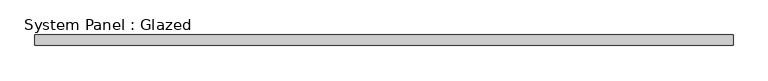
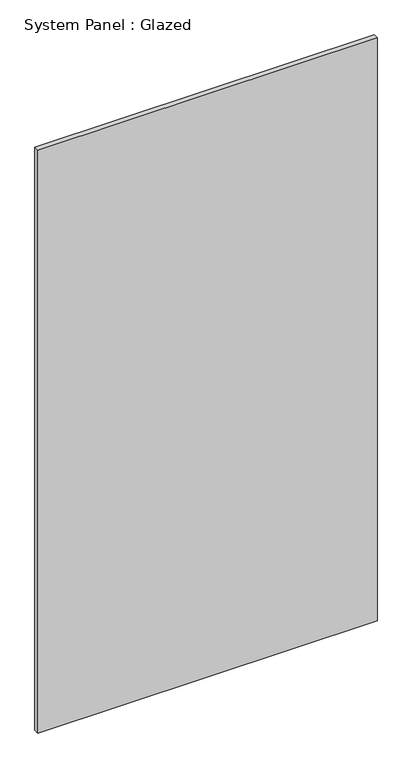
"""IFC4 building model written with IfcOpenShell, lengths in millimetres: plate geometry, System Panel : Glazed."""

from ifc_helpers import new_model, si_unit, origin, origin_with_axes, place, context, project, spatial, polyline, outline, extrude, source, transform, mapped, element, save


def system_panel_glazed_f5bfe384(model_context):
    return source(origin(), model_context, "Body", "SweptSolid", [
        extrude(outline(polyline([(825.6349237, 24.5), (-825.6349237, 24.5), (-825.6349237, 49.5), (825.6349237, 49.5), (825.6349237, 24.5)])), origin_with_axes(), (0.0, 0.0, 1.0), 3000.0),
    ])


if __name__ == "__main__":
    model = new_model("IFC4")
    model_context = context("Model", 3, world=origin())
    ifc_project = project(units=[si_unit("LENGTHUNIT", "METRE", prefix="MILLI")], contexts=[model_context])
    site = spatial("IfcSite", under=ifc_project)
    building = spatial("IfcBuilding", under=site)
    placement = place(None, origin())
    system_panel_glazed_shape = system_panel_glazed_f5bfe384(model_context)
    element("IfcPlate", 1, ObjectType="System Panel : Glazed", at=placement, inside=building, context=model_context, shape_type="MappedRepresentation", body=[
        mapped(system_panel_glazed_shape, transform((0.0, 0.0, 0.0), x_axis=(1.0, 0.0, 0.0), y_axis=(0.0, 1.0, 0.0), z_axis=(0.0, 0.0, 1.0))),
    ])
    save(model, "model.ifc")

# Revit data of these elements
# Type "System Panel : Glazed"
#   Keynote = "H11"
#   Construction Type Id = "GSP4R"
#   Analytic Construction = "1/8 in Pilkington single glazing"
#   Visual Light Transmittance = 0.9
#   Solar Heat Gain Coefficient = 0.86
#   Heat Transfer Coefficient (U) = 6.7069 W/(m²·K)
#   Define Thermal Properties by = 1
# Element 1 (IfcPlate, "System Panel : Glazed")
#   Materials on its faces: "Glass"
# Materials
#   "Glass": class "Glass", colour RGB 0 128 192, transparency 0.9, Description = "Soda Lime Glass", Cost = 0
